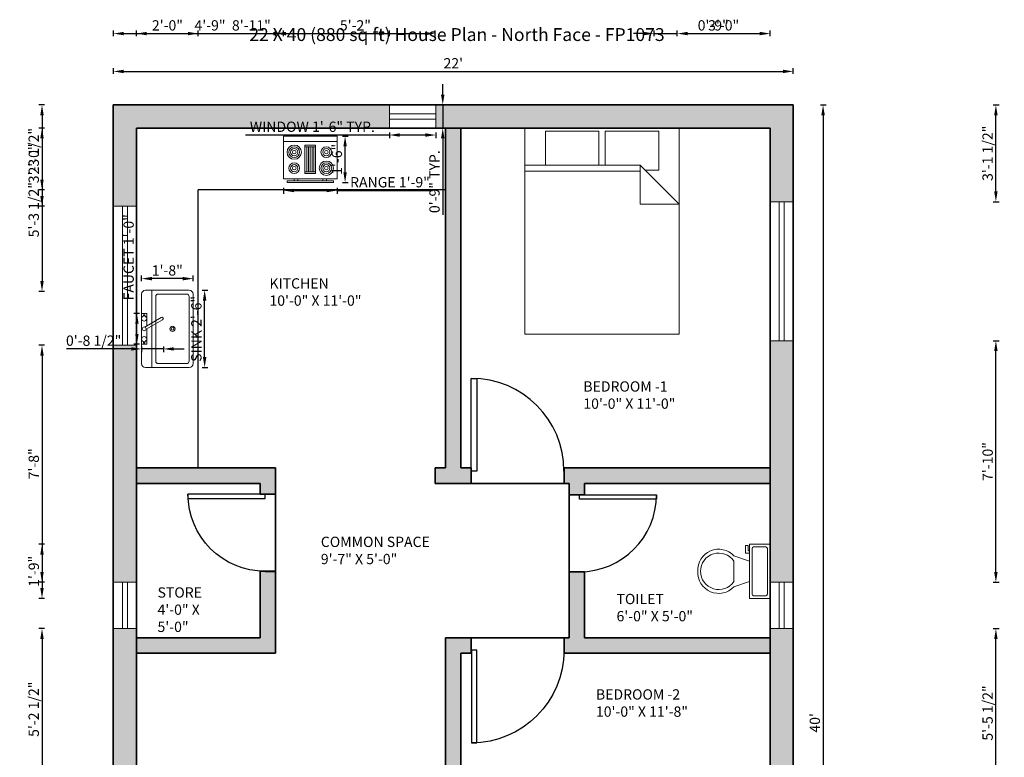
# Model space of a CAD drawing. Units: inches. Extents: x -34 to 348, y -513 to 46.
# Tile 2 of 2: x -34 to 348, y -240 to 46. Entities that reach past the tile are written whole.
import ezdxf

# ---------------------------------------------------------------- set-up
doc = ezdxf.new("R2010")
doc.units = ezdxf.units.IN
for name, color, linetype, lineweight in [('A-ANNO-DIMS', 2, 'Continuous', 18), ('A-ANNO-TEXT', 7, 'Continuous', 18), ('A-AREA-IDEN', 7, 'Continuous', 18), ('A-DOOR', 4, 'Continuous', 25), ('A-EQPM', 9, 'Continuous', 18), ('A-FLOR-CASE', 7, 'Continuous', 25), ('A-FLOR-FIXT', 8, 'Continuous', 18), ('A-FURN', 8, 'Continuous', 18), ('A-GLAZ', 6, 'Continuous', 18), ('A-WALL', 7, 'Continuous', 35), ('A-WALL-PATT', 251, 'Continuous', 13)]:
    doc.layers.add(name, color=color, linetype=linetype, lineweight=lineweight)
doc.styles.get("Standard").update_dxf_attribs({"font": 'arial.ttf'})
doc.dimstyles.new('ISO-25', dxfattribs={"dimtxt": 4, "dimasz": 4, "dimexe": 1.25, "dimexo": 0.625, "dimtad": 1, "dimlunit": 3, "dimtxsty": 'Standard', "dimcen": 2.5, "dimadec": 0, "dimazin": 0, "dimtfac": 1, "dimtmove": 0, "dimatfit": 3, "dimfxl": 1, "dimfxlon": 1, "dimarcsym": 0})

# ---------------------------------------------------------------- blocks, each defined once
blk = doc.blocks.new('*U2')
for p, q in [((9.5, -6), (9.5, -2)), ((-10, -8.5), (-8, -8.5)), ((-10, -9.5), (-10, -8.5)), ((-7, -9.5), (-10, -9.5)), ((-8, -8.5), (-8, -8)), ((-7, -8), (-7, -9.5)), ((-4, -8), (-6, -14)), ((4, -8), (6, -14)), ((4, -14), (-4, -14))]:
    blk.add_line(p, q)
blk.add_lwpolyline([(10.5, -8), (10.5, 0), (-10.5, 0), (-10.5, -8)], close=True)
for points in [[(-9.5, -2), (-9.5, -6)], [(8.5, -1), (-8.5, -1)], [(-8.5, -7), (8.5, -7)]]:
    blk.add_lwpolyline(points)
for centre, radius, start, end in [((-8.625, -1.875), 0.8839, 81.8699, 188.1301), ((8.625, -1.875), 0.8839, 351.8699, 98.1301), ((-8.625, -6.125), 0.8839, 171.869898, 278.1301), ((8.625, -6.125), 0.8839, 261.8699, 8.1301), ((-0.4772, -19.9188), 8.0953, 133.01722, 273.38), ((0.0374, -19.8731), 7.127, 124.50543, 269.7), ((-0.0373, -19.8731), 7.127, 270.3, 55.4946), ((0.4773, -19.9188), 8.0953, 266.62, 46.9828)]:
    blk.add_arc(centre, radius, start, end)
blk = doc.blocks.new('*U4')
for p, q in [((0, 0), (0, -100)), ((750, 0), (750, -100))]:
    blk.add_line(p, q)
blk.add_lwpolyline([(0, 0), (0, 750), (43.75, 750), (43.75, 0)], close=True)
blk.add_arc((0, 0), 750, 0, 90)
blk = doc.blocks.new('Sink-single - 30 in top')
blk.add_line((-15, -3.999996), (15, -3.999996))
for points in [[(-13.5, 0), (13.5, 0)], [(-15, -18.499996), (-15, -1.5)], [(15, -1.5), (15, -18.499996)], [(-13.5, -17.499996), (-13.5, -6.499996)], [(-12.5, -5.499996), (12.5, -5.499996)], [(13.5, -6.499996), (13.5, -17.499996)], [(12.5, -18.499996), (-12.5, -18.499996)], [(13.5, -19.999996), (-13.5, -19.999996)]]:
    blk.add_lwpolyline(points)
for radius in [1, 0.5]:
    blk.add_circle((0, -11.999996), radius)
for centre, radius, start, end in [((-13.5, -1.5), 1.5, 90, 180), ((13.5, -1.5), 1.5, 0, 90), ((-12.5, -6.499996), 1, 90, 180), ((12.5, -6.499996), 1, 0, 90), ((-13.5, -18.499996), 1.5, 180, 270), ((-12.5, -17.499996), 1, 180, 270), ((12.5, -17.499996), 1, 270, 0), ((13.5, -18.499996), 1.5, 270, 0)]:
    blk.add_arc(centre, radius, start, end)
blk = doc.blocks.new('Faucet - kit sink top')
for p, q in [((-5.5, -0.75), (-5.5, -1.25)), ((-4.94278, -0.75), (-5.5, -0.75)), ((-5.5, -1.25), (-4.94278, -1.25)), ((-0.14775, -1.7441), (3.56698, -8.1782)), ((4.43301, -7.6782), (0.71828, -1.2441)), ((4.94278, -0.75), (5.5, -0.75)), ((5.5, -1.25), (4.94278, -1.25)), ((5.5, -0.75), (5.5, -1.25))]:
    blk.add_line(p, q)
blk.add_lwpolyline([(-0.00587, -2), (-6, -2), (-6, 0), (6, 0), (6, -2), (1.15195, -2)])
for centre, radius in [((-4, -1), 1), ((4, -1), 1), ((0, -1), 0.75)]:
    blk.add_circle(centre, radius)
blk.add_arc((4, -7.9282), 0.5, 210, 30)
blk = doc.blocks.new('Range-Oven - 30 in top')
for p, q in [((0, -3), (30, -3)), ((12, -6), (18, -6)), ((13, -20), (13, -6)), ((14, -6), (14, -20)), ((15, -20), (15, -6)), ((16, -6), (16, -20)), ((17, -20), (17, -6)), ((18, -20), (12, -20)), ((6, -24), (6, -25)), ((8, -25), (8, -24)), ((22, -25), (22, -24)), ((24, -24), (24, -25))]:
    blk.add_line(p, q)
for points in [[(0, -24), (0, 0), (30, 0), (30, -24)], [(12, -21), (12, -5), (18, -5), (18, -21)], [(2, -26), (2, -25), (28, -25), (28, -26)]]:
    blk.add_lwpolyline(points, close=True)
for centre, radius in [((6, -9), 4), ((6, -9), 3), ((6, -9), 2), ((6, -9), 1), ((24, -9), 3), ((24, -9), 2), ((24, -9), 1), ((6, -18), 3), ((6, -18), 2), ((24, -18), 4), ((24, -18), 3), ((24, -18), 2), ((6, -18), 1), ((24, -18), 1)]:
    blk.add_circle(centre, radius)
blk = doc.blocks.new('Bed - Queen')
for p, q in [((0, -80.00003), (0, 0)), ((0, 0), (59.99999, 0)), ((59.99999, 0), (59.99999, -80.00003)), ((7.99999, -1.2), (28.79998, -1.2)), ((7.99999, -14.4), (7.99999, -1.2)), ((28.79998, -1.2), (28.79998, -14.4)), ((31.19999, -1.2), (51.99999, -1.2)), ((31.19999, -14.4), (31.19999, -1.2)), ((51.99999, -1.2), (51.99999, -16.4)), ((0, -14.4), (44.8, -14.4)), ((59.99999, -29.6), (44.8, -14.4)), ((44.8, -14.4), (44.8, -29.6)), ((44.8, -16.8), (0, -16.8)), ((51.99999, -16.4), (46.79936, -16.4)), ((44.8, -29.6), (59.99999, -29.6)), ((59.99999, -80.00003), (0, -80.00003))]:
    blk.add_line(p, q)
blk = doc.blocks.new('*D12')
at = {"layer": 'A-ANNO-DIMS', "color": 0, "lineweight": -2, "transparency": 16777216}
for p, q in [((2.13, 25.41), (2.13, 27.66)), ((266.13, 25.41), (266.13, 27.66)), ((6.13, 26.41), (262.13, 26.41))]:
    blk.add_line(p, q, dxfattribs=at)
at = {"layer": 'A-ANNO-DIMS', "color": 0, "transparency": 16777216}
for points in [[(6.13, 27.07), (6.13, 25.74), (2.13, 26.41)], [(262.13, 27.07), (262.13, 25.74), (266.13, 26.41)]]:
    blk.add_solid(points, dxfattribs=at)
at = {"layer": 'Defpoints', "color": 0, "transparency": 16777216}
for p in [(266.13, 26.41), (2.13, 13.4), (266.13, 13.4)]:
    blk.add_point(p, dxfattribs=at)
at = {"layer": 'A-ANNO-DIMS', "color": 0, "transparency": 16777216, "insert": (134.13, 29.04), "char_height": 4, "attachment_point": 5}
blk.add_mtext("22'", dxfattribs=at)
blk = doc.blocks.new('*D13')
at = {"layer": 'A-ANNO-DIMS', "color": 0, "lineweight": -2, "transparency": 16777216}
for p, q in [((276.72, 13.4), (278.97, 13.4)), ((277.72, 9.4), (277.72, -462.6)), ((276.72, -466.6), (278.97, -466.6))]:
    blk.add_line(p, q, dxfattribs=at)
at = {"layer": 'A-ANNO-DIMS', "color": 0, "transparency": 16777216}
for points in [[(277.06, 9.4), (278.39, 9.4), (277.72, 13.4)], [(277.06, -462.6), (278.39, -462.6), (277.72, -466.6)]]:
    blk.add_solid(points, dxfattribs=at)
at = {"layer": 'Defpoints', "color": 0, "transparency": 16777216}
for p in [(266.13, 13.4), (266.13, -466.6), (277.72, -466.6)]:
    blk.add_point(p, dxfattribs=at)
at = {"layer": 'A-ANNO-DIMS', "color": 0, "transparency": 16777216, "insert": (275.05, -226.6), "char_height": 4, "attachment_point": 5, "rotation": 90}
blk.add_mtext("40'", dxfattribs=at)
blk = doc.blocks.new('WIN-54IN')
for p, q in [((3.5, 54), (3.5, 0)), ((5.5, 54), (5.5, 0))]:
    blk.add_line(p, q)
blk.add_lwpolyline([(0, 54), (9, 54), (9, 0), (0, 0)], close=True)
blk = doc.blocks.new('WIN-18IN')
for p, q in [((3.5, 18), (3.5, 0)), ((5.5, 18), (5.5, 0))]:
    blk.add_line(p, q)
blk.add_lwpolyline([(0, 18), (9, 18), (9, 0), (0, 0)], close=True)
blk = doc.blocks.new('*D18')
at = {"layer": 'A-ANNO-DIMS', "color": 0, "lineweight": -2, "transparency": 16777216}
for p, q in [((109.34, 1.7), (53.47, 1.7)), ((109.34, 2.7), (109.34, 0.45)), ((123.34, 1.7), (113.34, 1.7)), ((127.34, 2.7), (127.34, 0.45))]:
    blk.add_line(p, q, dxfattribs=at)
at = {"layer": 'A-ANNO-DIMS', "color": 0, "transparency": 16777216}
for points in [[(113.34, 2.37), (113.34, 1.04), (109.34, 1.7)], [(123.34, 2.37), (123.34, 1.04), (127.34, 1.7)]]:
    blk.add_solid(points, dxfattribs=at)
at = {"layer": 'Defpoints', "color": 0, "transparency": 16777216}
for p in [(109.34, 4.4), (127.34, 4.4), (109.34, 1.7)]:
    blk.add_point(p, dxfattribs=at)
at = {"layer": 'A-ANNO-DIMS', "color": 0, "transparency": 16777216, "insert": (79.41, 4.4), "char_height": 4, "attachment_point": 5}
blk.add_mtext('WINDOW 1\'-6" TYP.', dxfattribs=at)
blk = doc.blocks.new('*D19')
at = {"layer": 'A-ANNO-DIMS', "color": 0, "lineweight": -2, "transparency": 16777216}
for p, q in [((130.04, 17.4), (130.04, 21.4)), ((129.04, 13.4), (131.29, 13.4)), ((130.04, 13.4), (130.04, 4.4)), ((129.04, 4.4), (131.29, 4.4)), ((130.04, 0.4), (130.04, -29.23))]:
    blk.add_line(p, q, dxfattribs=at)
at = {"layer": 'A-ANNO-DIMS', "color": 0, "transparency": 16777216}
for points in [[(129.37, 17.4), (130.71, 17.4), (130.04, 13.4)], [(129.37, 0.4), (130.71, 0.4), (130.04, 4.4)]]:
    blk.add_solid(points, dxfattribs=at)
at = {"layer": 'Defpoints', "color": 0, "transparency": 16777216}
for p in [(127.34, 13.4), (127.34, 4.4), (130.04, 4.4)]:
    blk.add_point(p, dxfattribs=at)
at = {"layer": 'A-ANNO-DIMS', "color": 0, "transparency": 16777216, "insert": (127.37, -16.41), "char_height": 4, "attachment_point": 5, "rotation": 90}
blk.add_mtext('0\'-9" TYP.', dxfattribs=at)
blk = doc.blocks.new('*D22')
at = {"layer": 'A-ANNO-DIMS', "color": 0, "lineweight": -2, "transparency": 16777216}
for p, q in [((36.58, -58.57), (38.83, -58.57)), ((37.58, -84.57), (37.58, -62.57)), ((36.58, -88.57), (38.83, -88.57))]:
    blk.add_line(p, q, dxfattribs=at)
at = {"layer": 'A-ANNO-DIMS', "color": 0, "transparency": 16777216}
for points in [[(36.92, -62.57), (38.25, -62.57), (37.58, -58.57)], [(36.92, -84.57), (38.25, -84.57), (37.58, -88.57)]]:
    blk.add_solid(points, dxfattribs=at)
at = {"layer": 'Defpoints', "color": 0, "transparency": 16777216}
for p in [(33.08, -58.57), (37.58, -58.57), (33.08, -88.57)]:
    blk.add_point(p, dxfattribs=at)
at = {"layer": 'A-ANNO-DIMS', "color": 0, "transparency": 16777216, "insert": (34.89, -73.57), "char_height": 4, "attachment_point": 5, "rotation": 90}
blk.add_mtext('SINK 2\'-6"', dxfattribs=at)
blk = doc.blocks.new('*D23')
at = {"layer": 'A-ANNO-DIMS', "color": 0, "lineweight": -2, "transparency": 16777216}
for p, q in [((13.08, -55.07), (13.08, -52.82)), ((33.08, -55.07), (33.08, -52.82)), ((29.08, -54.07), (17.08, -54.07))]:
    blk.add_line(p, q, dxfattribs=at)
at = {"layer": 'A-ANNO-DIMS', "color": 0, "transparency": 16777216}
for points in [[(17.08, -53.41), (17.08, -54.74), (13.08, -54.07)], [(29.08, -53.41), (29.08, -54.74), (33.08, -54.07)]]:
    blk.add_solid(points, dxfattribs=at)
at = {"layer": 'Defpoints', "color": 0, "transparency": 16777216}
for p in [(13.08, -54.07), (13.08, -58.57), (33.08, -58.57)]:
    blk.add_point(p, dxfattribs=at)
at = {"layer": 'A-ANNO-DIMS', "color": 0, "transparency": 16777216, "insert": (23.08, -51.41), "char_height": 4, "attachment_point": 5}
blk.add_mtext('1\'-8"', dxfattribs=at)
blk = doc.blocks.new('*D24')
at = {"layer": 'A-ANNO-DIMS', "color": 0, "lineweight": -2, "transparency": 16777216}
for p, q in [((11.28, -67.57), (11.28, -28.01)), ((12.28, -67.57), (10.03, -67.57)), ((11.28, -75.57), (11.28, -71.57)), ((12.28, -79.57), (10.03, -79.57))]:
    blk.add_line(p, q, dxfattribs=at)
at = {"layer": 'A-ANNO-DIMS', "color": 0, "transparency": 16777216}
for points in [[(10.62, -71.57), (11.95, -71.57), (11.28, -67.57)], [(10.62, -75.57), (11.95, -75.57), (11.28, -79.57)]]:
    blk.add_solid(points, dxfattribs=at)
at = {"layer": 'Defpoints', "color": 0, "transparency": 16777216}
for p in [(11.28, -67.57), (13.08, -67.57), (13.08, -79.57)]:
    blk.add_point(p, dxfattribs=at)
at = {"layer": 'A-ANNO-DIMS', "color": 0, "transparency": 16777216, "insert": (8.59, -45.79), "char_height": 4, "attachment_point": 5, "rotation": 90}
blk.add_mtext('FAUCET 1\'-0"', dxfattribs=at)
blk = doc.blocks.new('*D25')
at = {"layer": 'A-ANNO-DIMS', "color": 0, "lineweight": -2, "transparency": 16777216}
for p, q in [((9.08, -81.37), (-16.12, -81.37)), ((13.08, -80.37), (13.08, -82.62)), ((21.58, -81.37), (13.08, -81.37)), ((21.58, -80.37), (21.58, -82.62)), ((25.58, -81.37), (29.58, -81.37))]:
    blk.add_line(p, q, dxfattribs=at)
at = {"layer": 'A-ANNO-DIMS', "color": 0, "transparency": 16777216}
for points in [[(9.08, -80.71), (9.08, -82.04), (13.08, -81.37)], [(25.58, -80.71), (25.58, -82.04), (21.58, -81.37)]]:
    blk.add_solid(points, dxfattribs=at)
at = {"layer": 'Defpoints', "color": 0, "transparency": 16777216}
for p in [(13.08, -79.57), (21.58, -79.57), (13.08, -81.37)]:
    blk.add_point(p, dxfattribs=at)
at = {"layer": 'A-ANNO-DIMS', "color": 0, "transparency": 16777216, "insert": (-5.52, -78.68), "char_height": 4, "attachment_point": 5}
blk.add_mtext('0\'-8 1/2"', dxfattribs=at)
blk = doc.blocks.new('*D26')
at = {"layer": 'A-ANNO-DIMS', "color": 0, "lineweight": -2, "transparency": 16777216}
for p, q in [((68.22, -18.84), (68.22, -21.09)), ((89, -18.84), (89, -21.09)), ((72.22, -19.84), (85, -19.84)), ((89, -19.84), (126.1, -19.84))]:
    blk.add_line(p, q, dxfattribs=at)
at = {"layer": 'A-ANNO-DIMS', "color": 0, "transparency": 16777216}
for points in [[(72.22, -19.18), (72.22, -20.51), (68.22, -19.84)], [(85, -19.18), (85, -20.51), (89, -19.84)]]:
    blk.add_solid(points, dxfattribs=at)
at = {"layer": 'Defpoints', "color": 0, "transparency": 16777216}
for p in [(68.22, -16.73), (89, -16.73), (89, -19.84)]:
    blk.add_point(p, dxfattribs=at)
at = {"layer": 'A-ANNO-DIMS', "color": 0, "transparency": 16777216, "insert": (109.55, -17.15), "char_height": 4, "attachment_point": 5}
blk.add_mtext('RANGE 1\'-9"', dxfattribs=at)
blk = doc.blocks.new('*D27')
at = {"layer": 'A-ANNO-DIMS', "color": 0, "lineweight": -2, "transparency": 16777216}
for p, q in [((91.12, 1.29), (93.37, 1.29)), ((92.12, -12.73), (92.12, -2.71)), ((91.12, -16.73), (93.37, -16.73))]:
    blk.add_line(p, q, dxfattribs=at)
at = {"layer": 'A-ANNO-DIMS', "color": 0, "transparency": 16777216}
for points in [[(91.45, -2.71), (92.78, -2.71), (92.12, 1.29)], [(91.45, -12.73), (92.78, -12.73), (92.12, -16.73)]]:
    blk.add_solid(points, dxfattribs=at)
at = {"layer": 'Defpoints', "color": 0, "transparency": 16777216}
for p in [(89, 1.29), (92.12, 1.29), (89, -16.73)]:
    blk.add_point(p, dxfattribs=at)
at = {"layer": 'A-ANNO-DIMS', "color": 0, "transparency": 16777216, "insert": (89.45, -7.72), "char_height": 4, "attachment_point": 5, "rotation": 90}
blk.add_mtext('1\'-6"', dxfattribs=at)
blk = doc.blocks.new('*D33')
at = {"layer": 'A-ANNO-DIMS', "color": 0, "lineweight": -2, "transparency": 16777216}
for p, q in [((31.1, -510.8), (31.1, -513.05)), ((35.1, -511.8), (57.12, -511.8)), ((61.12, -510.8), (61.12, -513.05))]:
    blk.add_line(p, q, dxfattribs=at)
at = {"layer": 'A-ANNO-DIMS', "color": 0, "transparency": 16777216}
for points in [[(35.1, -511.13), (35.1, -512.47), (31.1, -511.8)], [(57.12, -511.13), (57.12, -512.47), (61.12, -511.8)]]:
    blk.add_solid(points, dxfattribs=at)
at = {"layer": 'Defpoints', "color": 0, "transparency": 16777216}
for p in [(31.1, -137.74), (61.12, -137.74), (61.12, -511.8)]:
    blk.add_point(p, dxfattribs=at)
at = {"layer": 'A-ANNO-DIMS', "color": 0, "transparency": 16777216, "insert": (46.11, -509.13), "char_height": 4, "attachment_point": 5}
blk.add_mtext('2\'-6"', dxfattribs=at)
blk = doc.blocks.new('*D34')
at = {"layer": 'A-ANNO-DIMS', "color": 0, "lineweight": -2, "transparency": 16777216}
for p, q in [((11.13, 40.1), (11.13, 42.35)), ((35.13, 40.1), (35.13, 42.35)), ((15.13, 41.1), (31.13, 41.1))]:
    blk.add_line(p, q, dxfattribs=at)
at = {"layer": 'A-ANNO-DIMS', "color": 0, "transparency": 16777216}
for points in [[(15.13, 41.77), (15.13, 40.44), (11.13, 41.1)], [(31.13, 41.77), (31.13, 40.44), (35.13, 41.1)]]:
    blk.add_solid(points, dxfattribs=at)
at = {"layer": 'Defpoints', "color": 0, "transparency": 16777216}
for p in [(35.13, 41.1), (11.13, -127.6), (35.13, -127.6)]:
    blk.add_point(p, dxfattribs=at)
at = {"layer": 'A-ANNO-DIMS', "color": 0, "transparency": 16777216, "insert": (23.13, 43.77), "char_height": 4, "attachment_point": 5}
blk.add_mtext('2\'-0"', dxfattribs=at)
blk = doc.blocks.new('*D35')
at = {"layer": 'A-ANNO-DIMS', "color": 0, "lineweight": -2, "transparency": 16777216}
for p, q in [((-24.57, 4.4), (-26.82, 4.4)), ((-25.57, 0.4), (-25.57, -15.6)), ((-24.57, -19.6), (-26.82, -19.6))]:
    blk.add_line(p, q, dxfattribs=at)
at = {"layer": 'A-ANNO-DIMS', "color": 0, "transparency": 16777216}
for points in [[(-26.24, 0.4), (-24.91, 0.4), (-25.57, 4.4)], [(-26.24, -15.6), (-24.91, -15.6), (-25.57, -19.6)]]:
    blk.add_solid(points, dxfattribs=at)
at = {"layer": 'Defpoints', "color": 0, "transparency": 16777216}
for p in [(131.13, 4.4), (-25.57, -19.6), (131.13, -19.6)]:
    blk.add_point(p, dxfattribs=at)
at = {"layer": 'A-ANNO-DIMS', "color": 0, "transparency": 16777216, "insert": (-28.24, -7.6), "char_height": 4, "attachment_point": 5, "rotation": 90}
blk.add_mtext('2\'-0"', dxfattribs=at)
blk = doc.blocks.new('*D36')
at = {"layer": 'A-ANNO-DIMS', "color": 0, "lineweight": -2, "transparency": 16777216}
for p, q in [((11.13, 40.1), (11.13, 42.35)), ((68.22, 40.1), (68.22, 42.35)), ((15.13, 41.1), (64.22, 41.1))]:
    blk.add_line(p, q, dxfattribs=at)
at = {"layer": 'A-ANNO-DIMS', "color": 0, "transparency": 16777216}
for points in [[(15.13, 41.77), (15.13, 40.44), (11.13, 41.1)], [(64.22, 41.77), (64.22, 40.44), (68.22, 41.1)]]:
    blk.add_solid(points, dxfattribs=at)
at = {"layer": 'Defpoints', "color": 0, "transparency": 16777216}
for p in [(68.22, 41.1), (11.13, 4.4), (68.22, 1.29)]:
    blk.add_point(p, dxfattribs=at)
at = {"layer": 'A-ANNO-DIMS', "color": 0, "transparency": 16777216, "insert": (39.67, 43.77), "char_height": 4, "attachment_point": 5}
blk.add_mtext('4\'-9"', dxfattribs=at)
blk = doc.blocks.new('*D37')
at = {"layer": 'A-ANNO-DIMS', "color": 0, "lineweight": -2, "transparency": 16777216}
for p, q in [((-24.57, 4.4), (-26.82, 4.4)), ((-25.57, 0.4), (-25.57, -55.01)), ((-24.57, -59.01), (-26.82, -59.01))]:
    blk.add_line(p, q, dxfattribs=at)
at = {"layer": 'A-ANNO-DIMS', "color": 0, "transparency": 16777216}
for points in [[(-26.24, 0.4), (-24.91, 0.4), (-25.57, 4.4)], [(-26.24, -55.01), (-24.91, -55.01), (-25.57, -59.01)]]:
    blk.add_solid(points, dxfattribs=at)
at = {"layer": 'Defpoints', "color": 0, "transparency": 16777216}
for p in [(11.13, 4.4), (-25.57, -59.01), (13.52, -59.01)]:
    blk.add_point(p, dxfattribs=at)
at = {"layer": 'A-ANNO-DIMS', "color": 0, "transparency": 16777216, "insert": (-28.27, -27.3), "char_height": 4, "attachment_point": 5, "rotation": 90}
blk.add_mtext('5\'-3 1/2"', dxfattribs=at)
blk = doc.blocks.new('*D38')
at = {"layer": 'A-ANNO-DIMS', "color": 0, "lineweight": -2, "transparency": 16777216}
for p, q in [((2.13, 40.1), (2.13, 42.35)), ((109.34, 40.1), (109.34, 42.35)), ((6.13, 41.1), (105.34, 41.1))]:
    blk.add_line(p, q, dxfattribs=at)
at = {"layer": 'A-ANNO-DIMS', "color": 0, "transparency": 16777216}
for points in [[(6.13, 41.77), (6.13, 40.44), (2.13, 41.1)], [(105.34, 41.77), (105.34, 40.44), (109.34, 41.1)]]:
    blk.add_solid(points, dxfattribs=at)
at = {"layer": 'Defpoints', "color": 0, "transparency": 16777216}
for p in [(109.34, 41.1), (2.13, 13.4), (109.34, 13.4)]:
    blk.add_point(p, dxfattribs=at)
at = {"layer": 'A-ANNO-DIMS', "color": 0, "transparency": 16777216, "insert": (55.73, 43.77), "char_height": 4, "attachment_point": 5}
blk.add_mtext('8\'-11"', dxfattribs=at)
blk = doc.blocks.new('*D39')
at = {"layer": 'A-ANNO-DIMS', "color": 0, "lineweight": -2, "transparency": 16777216}
for p, q in [((-24.57, 13.4), (-26.82, 13.4)), ((-25.57, 9.4), (-25.57, -21.97)), ((-24.57, -25.97), (-26.82, -25.97))]:
    blk.add_line(p, q, dxfattribs=at)
at = {"layer": 'A-ANNO-DIMS', "color": 0, "transparency": 16777216}
for points in [[(-26.24, 9.4), (-24.91, 9.4), (-25.57, 13.4)], [(-26.24, -21.97), (-24.91, -21.97), (-25.57, -25.97)]]:
    blk.add_solid(points, dxfattribs=at)
at = {"layer": 'Defpoints', "color": 0, "transparency": 16777216}
for p in [(2.13, 13.4), (-25.57, -25.97), (2.13, -25.97)]:
    blk.add_point(p, dxfattribs=at)
at = {"layer": 'A-ANNO-DIMS', "color": 0, "transparency": 16777216, "insert": (-28.27, -6.28), "char_height": 4, "attachment_point": 5, "rotation": 90}
blk.add_mtext('3\'-3 1/2"', dxfattribs=at)
blk = doc.blocks.new('*D40')
at = {"layer": 'A-ANNO-DIMS', "color": 0, "lineweight": -2, "transparency": 16777216}
for p, q in [((-24.57, -79.97), (-26.82, -79.97)), ((-25.57, -83.97), (-25.57, -168.01)), ((-24.57, -172.01), (-26.82, -172.01))]:
    blk.add_line(p, q, dxfattribs=at)
at = {"layer": 'A-ANNO-DIMS', "color": 0, "transparency": 16777216}
for points in [[(-26.24, -83.97), (-24.91, -83.97), (-25.57, -79.97)], [(-26.24, -168.01), (-24.91, -168.01), (-25.57, -172.01)]]:
    blk.add_solid(points, dxfattribs=at)
at = {"layer": 'Defpoints', "color": 0, "transparency": 16777216}
for p in [(2.13, -79.97), (-25.57, -172.01), (2.13, -172.01)]:
    blk.add_point(p, dxfattribs=at)
at = {"layer": 'A-ANNO-DIMS', "color": 0, "transparency": 16777216, "insert": (-28.24, -125.99), "char_height": 4, "attachment_point": 5, "rotation": 90}
blk.add_mtext('7\'-8"', dxfattribs=at)
blk = doc.blocks.new('*D41')
at = {"layer": 'A-ANNO-DIMS', "color": 0, "lineweight": -2, "transparency": 16777216}
for p, q in [((-24.57, -190.01), (-26.82, -190.01)), ((-25.57, -194.01), (-25.57, -248.61)), ((-24.57, -252.61), (-26.82, -252.61))]:
    blk.add_line(p, q, dxfattribs=at)
at = {"layer": 'A-ANNO-DIMS', "color": 0, "transparency": 16777216}
for points in [[(-26.24, -194.01), (-24.91, -194.01), (-25.57, -190.01)], [(-26.24, -248.61), (-24.91, -248.61), (-25.57, -252.61)]]:
    blk.add_solid(points, dxfattribs=at)
at = {"layer": 'Defpoints', "color": 0, "transparency": 16777216}
for p in [(2.13, -190.01), (-25.57, -252.61), (2.13, -252.61)]:
    blk.add_point(p, dxfattribs=at)
at = {"layer": 'A-ANNO-DIMS', "color": 0, "transparency": 16777216, "insert": (-28.27, -221.31), "char_height": 4, "attachment_point": 5, "rotation": 90}
blk.add_mtext('5\'-2 1/2"', dxfattribs=at)
blk = doc.blocks.new('*D43')
at = {"layer": 'A-ANNO-DIMS', "color": 0, "lineweight": -2, "transparency": 16777216}
for p, q in [((343.83, 13.4), (346.08, 13.4)), ((344.83, -20.18), (344.83, 9.4)), ((343.83, -24.18), (346.08, -24.18))]:
    blk.add_line(p, q, dxfattribs=at)
at = {"layer": 'A-ANNO-DIMS', "color": 0, "transparency": 16777216}
for points in [[(344.16, 9.4), (345.49, 9.4), (344.83, 13.4)], [(344.16, -20.18), (345.49, -20.18), (344.83, -24.18)]]:
    blk.add_solid(points, dxfattribs=at)
at = {"layer": 'Defpoints', "color": 0, "transparency": 16777216}
for p in [(266.13, 13.4), (344.83, 13.4), (266.13, -24.18)]:
    blk.add_point(p, dxfattribs=at)
at = {"layer": 'A-ANNO-DIMS', "color": 0, "transparency": 16777216, "insert": (342.13, -5.39), "char_height": 4, "attachment_point": 5, "rotation": 90}
blk.add_mtext('3\'-1 1/2"', dxfattribs=at)
blk = doc.blocks.new('*D44')
at = {"layer": 'A-ANNO-DIMS', "color": 0, "lineweight": -2, "transparency": 16777216}
for p, q in [((343.83, -78.18), (346.08, -78.18)), ((344.83, -168.01), (344.83, -82.18)), ((343.83, -172.01), (346.08, -172.01))]:
    blk.add_line(p, q, dxfattribs=at)
at = {"layer": 'A-ANNO-DIMS', "color": 0, "transparency": 16777216}
for points in [[(344.16, -82.18), (345.49, -82.18), (344.83, -78.18)], [(344.16, -168.01), (345.49, -168.01), (344.83, -172.01)]]:
    blk.add_solid(points, dxfattribs=at)
at = {"layer": 'Defpoints', "color": 0, "transparency": 16777216}
for p in [(266.13, -78.18), (344.83, -78.18), (266.13, -172.01)]:
    blk.add_point(p, dxfattribs=at)
at = {"layer": 'A-ANNO-DIMS', "color": 0, "transparency": 16777216, "insert": (342.16, -125.1), "char_height": 4, "attachment_point": 5, "rotation": 90}
blk.add_mtext('7\'-10"', dxfattribs=at)
blk = doc.blocks.new('*D45')
at = {"layer": 'A-ANNO-DIMS', "color": 0, "lineweight": -2, "transparency": 16777216}
for p, q in [((343.83, -190.01), (346.08, -190.01)), ((344.83, -251.53), (344.83, -194.01)), ((343.83, -255.53), (346.08, -255.53))]:
    blk.add_line(p, q, dxfattribs=at)
at = {"layer": 'A-ANNO-DIMS', "color": 0, "transparency": 16777216}
for points in [[(344.16, -194.01), (345.49, -194.01), (344.83, -190.01)], [(344.16, -251.53), (345.49, -251.53), (344.83, -255.53)]]:
    blk.add_solid(points, dxfattribs=at)
at = {"layer": 'Defpoints', "color": 0, "transparency": 16777216}
for p in [(266.13, -190.01), (344.83, -190.01), (266.13, -255.53)]:
    blk.add_point(p, dxfattribs=at)
at = {"layer": 'A-ANNO-DIMS', "color": 0, "transparency": 16777216, "insert": (342.13, -222.77), "char_height": 4, "attachment_point": 5, "rotation": 90}
blk.add_mtext('5\'-5 1/2"', dxfattribs=at)
blk = doc.blocks.new('*D48')
at = {"layer": 'A-ANNO-DIMS', "color": 0, "lineweight": -2, "transparency": 16777216}
for p, q in [((-24.57, -157.24), (-26.82, -157.24)), ((-25.57, -161.24), (-25.57, -174.24)), ((-24.57, -178.24), (-26.82, -178.24))]:
    blk.add_line(p, q, dxfattribs=at)
at = {"layer": 'A-ANNO-DIMS', "color": 0, "transparency": 16777216}
for points in [[(-26.24, -161.24), (-24.91, -161.24), (-25.57, -157.24)], [(-26.24, -174.24), (-24.91, -174.24), (-25.57, -178.24)]]:
    blk.add_solid(points, dxfattribs=at)
at = {"layer": 'Defpoints', "color": 0, "transparency": 16777216}
for p in [(249.13, -157.24), (-25.57, -178.24), (249.13, -178.24)]:
    blk.add_point(p, dxfattribs=at)
at = {"layer": 'A-ANNO-DIMS', "color": 0, "transparency": 16777216, "insert": (-28.24, -167.74), "char_height": 4, "attachment_point": 5, "rotation": 90}
blk.add_mtext('1\'-9"', dxfattribs=at)
blk = doc.blocks.new('*D49')
at = {"layer": 'A-ANNO-DIMS', "color": 0, "lineweight": -2, "transparency": 16777216}
for p, q in [((229.13, -510.8), (229.13, -513.05)), ((233.13, -511.8), (253.13, -511.8)), ((257.13, -510.8), (257.13, -513.05))]:
    blk.add_line(p, q, dxfattribs=at)
at = {"layer": 'A-ANNO-DIMS', "color": 0, "transparency": 16777216}
for points in [[(233.13, -511.13), (233.13, -512.47), (229.13, -511.8)], [(253.13, -511.13), (253.13, -512.47), (257.13, -511.8)]]:
    blk.add_solid(points, dxfattribs=at)
at = {"layer": 'Defpoints', "color": 0, "transparency": 16777216}
for p in [(229.13, -167.74), (257.13, -178.24), (257.13, -511.8)]:
    blk.add_point(p, dxfattribs=at)
at = {"layer": 'A-ANNO-DIMS', "color": 0, "transparency": 16777216, "insert": (243.13, -509.17), "char_height": 4, "attachment_point": 5}
blk.add_mtext('2\'-4"', dxfattribs=at)
blk = doc.blocks.new('*D50')
at = {"layer": 'A-ANNO-DIMS', "color": 0, "lineweight": -2, "transparency": 16777216}
for p, q in [((221.89, -510.8), (221.89, -513.05)), ((225.89, -511.8), (253.13, -511.8)), ((257.13, -510.8), (257.13, -513.05))]:
    blk.add_line(p, q, dxfattribs=at)
at = {"layer": 'A-ANNO-DIMS', "color": 0, "transparency": 16777216}
for points in [[(225.89, -511.13), (225.89, -512.47), (221.89, -511.8)], [(253.13, -511.13), (253.13, -512.47), (257.13, -511.8)]]:
    blk.add_solid(points, dxfattribs=at)
at = {"layer": 'Defpoints', "color": 0, "transparency": 16777216}
for p in [(221.89, 4.4), (257.13, 4.4), (257.13, -511.8)]:
    blk.add_point(p, dxfattribs=at)
at = {"layer": 'A-ANNO-DIMS', "color": 0, "transparency": 16777216, "insert": (239.51, -509.17), "char_height": 4, "attachment_point": 5}
blk.add_mtext('2\'-11"', dxfattribs=at)
blk = doc.blocks.new('*D51')
at = {"layer": 'A-ANNO-DIMS', "color": 0, "lineweight": -2, "transparency": 16777216}
for p, q in [((221.13, 40.1), (221.13, 42.35)), ((257.13, 40.1), (257.13, 42.35)), ((225.13, 41.1), (253.13, 41.1))]:
    blk.add_line(p, q, dxfattribs=at)
at = {"layer": 'A-ANNO-DIMS', "color": 0, "transparency": 16777216}
for points in [[(225.13, 41.77), (225.13, 40.44), (221.13, 41.1)], [(253.13, 41.77), (253.13, 40.44), (257.13, 41.1)]]:
    blk.add_solid(points, dxfattribs=at)
at = {"layer": 'Defpoints', "color": 0, "transparency": 16777216}
for p in [(257.13, 41.1), (221.13, -343.93), (257.13, -343.93)]:
    blk.add_point(p, dxfattribs=at)
at = {"layer": 'A-ANNO-DIMS', "color": 0, "transparency": 16777216, "insert": (239.13, 43.77), "char_height": 4, "attachment_point": 5}
blk.add_mtext('3\'-0"', dxfattribs=at)
blk = doc.blocks.new('*D52')
at = {"layer": 'A-ANNO-DIMS', "color": 0, "lineweight": -2, "transparency": 16777216}
for p, q in [((65.13, 40.1), (65.13, 42.35)), ((127.13, 40.1), (127.13, 42.35)), ((69.13, 41.1), (123.13, 41.1))]:
    blk.add_line(p, q, dxfattribs=at)
at = {"layer": 'A-ANNO-DIMS', "color": 0, "transparency": 16777216}
for points in [[(69.13, 41.77), (69.13, 40.44), (65.13, 41.1)], [(123.13, 41.77), (123.13, 40.44), (127.13, 41.1)]]:
    blk.add_solid(points, dxfattribs=at)
at = {"layer": 'Defpoints', "color": 0, "transparency": 16777216}
for p in [(127.13, 41.1), (65.13, -127.6), (127.13, -127.6)]:
    blk.add_point(p, dxfattribs=at)
at = {"layer": 'A-ANNO-DIMS', "color": 0, "transparency": 16777216, "insert": (96.13, 43.77), "char_height": 4, "attachment_point": 5}
blk.add_mtext('5\'-2"', dxfattribs=at)
blk = doc.blocks.new('*D53')
at = {"layer": 'A-ANNO-DIMS', "color": 0, "lineweight": -2, "transparency": 16777216}
for p, q in [((212.09, 40.1), (212.09, 42.35)), ((221.13, 40.1), (221.13, 42.35)), ((208.09, 41.1), (204.09, 41.1)), ((212.09, 41.1), (221.13, 41.1)), ((225.13, 41.1), (241.01, 41.1))]:
    blk.add_line(p, q, dxfattribs=at)
at = {"layer": 'A-ANNO-DIMS', "color": 0, "transparency": 16777216}
for points in [[(208.09, 41.77), (208.09, 40.44), (212.09, 41.1)], [(225.13, 41.77), (225.13, 40.44), (221.13, 41.1)]]:
    blk.add_solid(points, dxfattribs=at)
at = {"layer": 'Defpoints', "color": 0, "transparency": 16777216}
for p in [(221.13, 41.1), (212.09, -343.93), (221.13, -343.93)]:
    blk.add_point(p, dxfattribs=at)
at = {"layer": 'A-ANNO-DIMS', "color": 0, "transparency": 16777216, "insert": (235.07, 43.77), "char_height": 4, "attachment_point": 5}
blk.add_mtext('0\'-9"', dxfattribs=at)

msp = doc.modelspace()

# ---------------------------------------------------------------- hatches: boundary and pattern name
at = {"layer": 'A-WALL-PATT'}
h = msp.add_hatch(color=256, dxfattribs=at)
h.dxf.hatch_style = 1
h.paths.add_polyline_path([(109.341, 13.405), (2.127, 13.405), (2.127, -25.971), (11.127, -25.971), (11.127, 4.405), (109.341, 4.405)])
h.paths.add_polyline_path([(266.127, 13.405), (127.341, 13.405), (127.341, 4.405), (131.127, 4.405), (137.127, 4.405), (257.127, 4.405), (257.127, -24.182), (266.127, -24.182)])
h.paths.add_polyline_path([(11.127, -79.971), (2.127, -79.971), (2.127, -172.013), (11.127, -172.013)])
h.paths.add_polyline_path([(65.127, -127.595), (11.127, -127.595), (11.127, -133.595), (59.127, -133.595), (59.127, -137.743), (61.124, -137.743), (65.127, -137.743), (65.127, -133.595)])
h.paths.add_polyline_path([(65.127, -167.764), (61.124, -167.764, -0.0092932), (60.008, -167.743), (59.127, -167.743), (59.127, -193.595), (11.127, -193.595), (11.127, -199.595), (59.127, -199.595), (65.127, -199.595)])
h.paths.add_polyline_path([(11.127, -190.013), (2.127, -190.013), (2.127, -252.614), (11.127, -252.614)])
h.paths.add_polyline_path([(11.127, -306.614), (2.127, -306.614), (2.127, -388.939), (11.127, -388.939)])
h.paths.add_polyline_path([(85.316, -461.006), (85.316, -460.595), (11.127, -460.595), (11.127, -466.595), (85.316, -466.595)])
h.paths.add_polyline_path([(11.127, -442.939), (2.127, -442.939), (2.127, -466.595), (11.127, -466.595)])
h.paths.add_polyline_path([(137.127, -427.93), (257.127, -427.93), (257.127, -421.93), (131.127, -421.93), (125.127, -421.93), (125.127, -427.93), (131.127, -427.93), (131.127, -460.595), (127.316, -460.595), (127.316, -466.595), (132.166, -466.595), (137.127, -466.595)])
h.paths.add_polyline_path([(266.127, -394.659), (257.127, -394.659), (257.127, -421.93), (257.127, -427.93), (266.127, -427.93)])
h.paths.add_polyline_path([(266.127, -309.532), (257.127, -309.532), (257.127, -343.93), (257.127, -360.659), (266.127, -360.659)])
h.paths.add_polyline_path([(257.127, -338.93), (137.127, -338.93), (137.127, -199.595), (141.127, -199.595), (141.127, -193.595), (131.127, -193.595), (131.127, -338.93), (127.127, -338.93), (127.127, -339.114), (127.127, -343.93), (137.127, -343.93), (257.127, -343.93)])
h.paths.add_polyline_path([(91.006, -338.93), (11.127, -338.93), (11.127, -343.93), (91.006, -343.93)])
h.paths.add_polyline_path([(266.127, -190.013), (257.127, -190.013), (257.127, -255.532), (266.127, -255.532)])
h.paths.add_polyline_path([(257.127, -193.595), (185.127, -193.595), (185.127, -167.989), (179.127, -167.989), (179.127, -193.595), (177.136, -193.595), (177.136, -198.391, -0.0057168), (177.127, -199.214), (177.127, -199.595), (179.127, -199.595), (185.127, -199.595), (257.127, -199.595)])
h.paths.add_polyline_path([(266.127, -78.182), (257.127, -78.182), (257.127, -172.013), (266.127, -172.013)])
h.paths.add_polyline_path([(257.127, -127.595), (177.127, -127.595), (177.127, -133.595), (179.127, -133.595), (179.127, -137.989), (183.118, -137.989), (185.127, -137.989), (185.127, -133.595), (257.127, -133.595)])
h.paths.add_polyline_path([(137.127, 4.405), (131.127, 4.405), (131.127, -127.595), (127.127, -127.595), (127.127, -133.595), (131.127, -133.595), (137.127, -133.595), (141.127, -133.595), (141.127, -128.797), (141.127, -127.595), (137.127, -127.595)])

# ---------------------------------------------------------------- linework, layer by layer
at = {"layer": 'A-FLOR-CASE'}
for p in [(131.127, -19.595), (35.127, -127.595)]:
    msp.add_line(p, (35.127, -19.595), dxfattribs=at)
at = {"layer": 'A-WALL'}
for p, q in [((2.127, 13.405), (266.127, 13.405)), ((2.127, -466.595), (2.127, 13.405)), ((266.127, 13.405), (266.127, -427.93)), ((11.127, 4.405), (131.127, 4.405)), ((11.127, -466.595), (11.127, 4.405)), ((131.127, 4.405), (137.127, 4.405)), ((131.127, -127.595), (131.127, 4.405)), ((137.127, 4.405), (257.127, 4.405)), ((137.127, -127.595), (137.127, 4.405)), ((257.127, 4.405), (257.127, -343.93)), ((11.127, -127.595), (65.127, -127.595)), ((65.127, -133.595), (65.127, -127.595)), ((127.127, -127.595), (127.127, -133.595)), ((127.127, -127.595), (131.127, -127.595)), ((137.127, -127.595), (141.127, -127.595)), ((141.127, -127.595), (141.127, -133.595)), ((177.127, -127.595), (177.127, -133.595)), ((177.127, -127.595), (257.127, -127.595)), ((11.127, -133.595), (59.127, -133.595)), ((59.127, -133.595), (59.127, -137.743)), ((65.127, -133.595), (65.127, -199.595)), ((127.127, -133.595), (131.127, -133.595)), ((137.127, -133.595), (131.127, -133.595)), ((137.127, -133.595), (179.127, -133.595)), ((179.127, -133.595), (179.127, -193.595)), ((185.127, -133.595), (185.127, -137.989)), ((185.127, -133.595), (257.127, -133.595)), ((65.127, -137.743), (59.127, -137.743)), ((185.127, -137.989), (179.127, -137.989)), ((65.127, -167.743), (59.127, -167.743)), ((59.127, -167.743), (59.127, -193.595)), ((185.127, -167.989), (179.127, -167.989)), ((185.127, -167.989), (185.127, -193.595)), ((59.127, -193.595), (11.127, -193.595)), ((179.127, -193.595), (131.127, -193.595)), ((131.127, -338.93), (131.127, -193.595)), ((141.127, -199.595), (141.127, -193.595)), ((177.127, -199.595), (177.127, -193.595)), ((185.127, -193.595), (257.127, -193.595)), ((59.127, -199.595), (11.127, -199.595)), ((59.127, -199.595), (65.127, -199.595)), ((141.127, -199.595), (137.127, -199.595)), ((137.127, -338.93), (137.127, -199.595)), ((179.127, -199.595), (177.127, -199.595)), ((185.127, -199.595), (179.127, -199.595)), ((185.127, -199.595), (257.127, -199.595))]:
    msp.add_line(p, q, dxfattribs=at)

# ---------------------------------------------------------------- block references
at = {"layer": 'A-DOOR', "xscale": 0.0479834075053935, "yscale": 0.0479834075053935, "zscale": 0.0479834075053935}
msp.add_blockref('*U4', (141.127, -128.797), dxfattribs=at)
at = {"layer": 'A-DOOR'}
for p, xscale, yscale, zscale, rotation in [((61.124, -137.743), -0.040027650715538, 0.040027650715538, 0.040027650715538, 90), ((183.118, -137.989), 0.0399172122118605, 0.0399172122118605, 0.0399172122118605, 270), ((141.142, -198.391), -0.0479923476985897, 0.0479923476985897, 0.0479923476985897, 180)]:
    msp.add_blockref('*U4', p, dxfattribs=dict(at, xscale=xscale, yscale=yscale, zscale=zscale, rotation=rotation))
at = {"layer": 'A-EQPM', "xscale": 0.6928203345745566, "yscale": 0.6928203345745566, "zscale": 0.6928203345745566}
msp.add_blockref('Range-Oven - 30 in top', (68.215, 1.287), dxfattribs=at)
at = {"layer": 'A-FLOR-FIXT'}
for name, p, rotation in [('Sink-single - 30 in top', (13.082, -73.575), 90), ('Faucet - kit sink top', (13.082, -73.575), 90), ('*U2', (257.127, -167.738), 270)]:
    msp.add_blockref(name, p, dxfattribs=dict(at, rotation=rotation))
at = {"layer": 'A-FURN'}
msp.add_blockref('Bed - Queen', (161.891, 4.405), dxfattribs=at)
at = {"layer": 'A-GLAZ', "extrusion": (0, 0, -1), "zscale": -1, "rotation": 270.0000000000002}
msp.add_blockref('WIN-18IN', (-127.341, 13.405), dxfattribs=at)
at = {"layer": 'A-GLAZ'}
for name, p in [('WIN-54IN', (2.127, -79.971)), ('WIN-54IN', (257.127, -78.182)), ('WIN-18IN', (2.127, -190.013)), ('WIN-18IN', (257.127, -190.013))]:
    msp.add_blockref(name, p, dxfattribs=at)

# ---------------------------------------------------------------- texts
at = {"layer": 'A-ANNO-TEXT', "insert": (54.926, 43.219), "char_height": 5, "attachment_point": 1}
msp.add_mtext_dynamic_manual_height_columns('22 X 40 (880 sq ft) House Plan - North Face - FP1073', width=228.37722, gutter_width=12.5, heights=[0], dxfattribs=at)
at = {"layer": 'A-AREA-IDEN', "char_height": 4, "attachment_point": 1}
for s, width, insert in [('KITCHEN\\P10\'-0" X 11\'-0"', 64.44418, (62.748, -53.933)), ('BEDROOM -1\\P10\'-0" X 11\'-0"', 61.1625, (184.634, -93.956)), ('COMMON SPACE\\P9\'-7" X 5\'-0"', 82.73794, (82.701, -154.301)), ('STORE\\P4\'-0" X 5\'-0"', 29.61025, (19.288, -173.973)), ('TOILET\\P6\'-0" X 5\'-0"', 30.90505, (197.522, -176.499)), ('BEDROOM -2\\P10\'-0" X 11\'-8"', 51.47015, (189.53, -213.565))]:
    msp.add_mtext_dynamic_manual_height_columns(s, width=width, gutter_width=12.5, heights=[0], dxfattribs=dict(at, insert=insert))

# ---------------------------------------------------------------- dimensions: what is measured, and where the dimension line sits
at = {"layer": 'A-ANNO-DIMS'}
for base, p1, p2, override, picture, middle in [((109.341, 41.105), (2.127, 13.405), (109.341, 13.405), {"dimdec": 1, "dimlfac": 1, "dimrnd": 0, "dimzin": 1, "dimdsep": 46, "dimlunit": 4, "dimfrac": 2}, '*D38', (55.734, 43.772)), ((35.127, 41.105), (11.127, -127.595), (35.127, -127.595), {"dimdec": 1, "dimlfac": 1, "dimrnd": 0, "dimzin": 1, "dimdsep": 46, "dimlunit": 4, "dimfrac": 2}, '*D34', (23.127, 43.772)), ((68.215, 41.105), (11.127, 4.405), (68.215, 1.287), {"dimdec": 1, "dimlfac": 1, "dimrnd": 0, "dimzin": 1, "dimdsep": 46, "dimlunit": 4, "dimfrac": 2}, '*D36', (39.671, 43.772)), ((127.127, 41.105), (65.127, -127.595), (127.127, -127.595), {"dimdec": 1, "dimlfac": 1, "dimrnd": 0, "dimzin": 1, "dimdsep": 46, "dimlunit": 4, "dimfrac": 2}, '*D52', (96.127, 43.772)), ((221.127, 41.105), (212.094, -343.93), (221.127, -343.93), {"dimdec": 1, "dimlfac": 1, "dimrnd": 0, "dimzin": 1, "dimdsep": 46, "dimlunit": 4, "dimfrac": 2}, '*D53', (235.068, 43.772)), ((257.127, 41.105), (221.127, -343.93), (257.127, -343.93), {"dimdec": 1, "dimlfac": 1, "dimrnd": 0, "dimzin": 1, "dimdsep": 46, "dimlunit": 4, "dimfrac": 2}, '*D51', (239.127, 43.773)), ((266.127, 26.405), (2.127, 13.405), (266.127, 13.405), {"dimclrd": 0, "dimclre": 0, "dimclrt": 0}, '*D12', (134.127, 29.038)), ((257.127, -511.8), (221.891, 4.405), (257.127, 4.405), {"dimdec": 1, "dimlfac": 1, "dimrnd": 0, "dimzin": 1, "dimdsep": 46, "dimlunit": 4, "dimfrac": 2}, '*D50', (239.509, -509.166)), ((61.124, -511.8), (31.103, -137.743), (61.124, -137.743), {"dimdec": 1, "dimlfac": 1, "dimrnd": 0, "dimzin": 1, "dimdsep": 46, "dimlunit": 4, "dimfrac": 2}, '*D33', (46.114, -509.132)), ((257.127, -511.8), (229.127, -167.738), (257.127, -178.238), {"dimdec": 1, "dimlfac": 1, "dimrnd": 0, "dimzin": 1, "dimdsep": 46, "dimlunit": 4, "dimfrac": 2}, '*D49', (243.127, -509.166))]:
    dim = msp.add_linear_dim(base=base, p1=p1, p2=p2, dimstyle='ISO-25', override=override, dxfattribs=at)
    dim.commit()
    dim.dimension.update_dxf_attribs({"geometry": picture, "text_midpoint": middle})
for base, p1, p2, angle, text, picture, middle in [((130.041, 4.405), (127.341, 13.405), (127.341, 4.405), 270, '<> TYP.', '*D19', (127.374, -16.411)), ((109.341, 1.705), (127.341, 4.405), (109.341, 4.405), 180, 'WINDOW <> TYP.', '*D18', (79.408, 4.399)), ((11.282, -67.575), (13.082, -79.575), (13.082, -67.575), 90, 'FAUCET <>', '*D24', (8.589, -45.794)), ((37.582, -58.575), (33.082, -88.575), (33.082, -58.575), 90, 'SINK <>', '*D22', (34.889, -73.575))]:
    dim = msp.add_linear_dim(base=base, p1=p1, p2=p2, angle=angle, text=text, dimstyle='ISO-25', override={"dimdec": 1, "dimlfac": 1, "dimrnd": 0, "dimzin": 1, "dimdsep": 46, "dimlunit": 4, "dimfrac": 2}, dxfattribs=at)
    dim.commit()
    dim.dimension.update_dxf_attribs({"geometry": picture, "text_midpoint": middle})
for base, p1, p2, angle, picture, middle in [((-25.573, -25.971), (2.127, 13.405), (2.127, -25.971), 90, '*D39', (-28.268, -6.283)), ((344.827, 13.405), (266.127, -24.182), (266.127, 13.405), 90, '*D43', (342.132, -5.389)), ((-25.573, -59.014), (11.127, 4.405), (13.521, -59.014), 90, '*D37', (-28.268, -27.305)), ((-25.573, -19.595), (131.127, 4.405), (131.127, -19.595), 90, '*D35', (-28.241, -7.595)), ((92.118, 1.287), (89, -16.727), (89, 1.287), 90, '*D27', (89.45, -7.72)), ((13.082, -54.075), (33.082, -58.575), (13.082, -58.575), 180, '*D23', (23.082, -51.407)), ((13.082, -81.375), (21.581, -79.575), (13.082, -79.575), 180, '*D25', (-5.52, -78.681)), ((-25.573, -172.013), (2.127, -79.971), (2.127, -172.013), 90, '*D40', (-28.241, -125.992)), ((344.827, -78.182), (266.127, -172.013), (266.127, -78.182), 90, '*D44', (342.159, -125.097)), ((-25.573, -178.238), (249.127, -157.238), (249.127, -178.238), 90, '*D48', (-28.241, -167.738)), ((-25.573, -252.614), (2.127, -190.013), (2.127, -252.614), 90, '*D41', (-28.266, -221.313)), ((344.827, -190.013), (266.127, -255.532), (266.127, -190.013), 90, '*D45', (342.134, -222.772))]:
    dim = msp.add_linear_dim(base=base, p1=p1, p2=p2, angle=angle, dimstyle='ISO-25', override={"dimdec": 1, "dimlfac": 1, "dimrnd": 0, "dimzin": 1, "dimdsep": 46, "dimlunit": 4, "dimfrac": 2}, dxfattribs=at)
    dim.commit()
    dim.dimension.update_dxf_attribs({"geometry": picture, "text_midpoint": middle})
dim = msp.add_linear_dim(base=(277.722, -466.595), p1=(266.127, 13.405), p2=(266.127, -466.595), angle=90, dimstyle='ISO-25', override={"dimclrd": 0, "dimclre": 0, "dimclrt": 0}, dxfattribs=at)
dim.commit()
dim.dimension.update_dxf_attribs({"geometry": '*D13', "text_midpoint": (277.722, -226.595), "dimtype": 160})
dim = msp.add_linear_dim(base=(89, -19.844), p1=(68.215, -16.727), p2=(89, -16.727), text='RANGE <>', dimstyle='ISO-25', override={"dimdec": 1, "dimlfac": 1, "dimrnd": 0, "dimzin": 1, "dimdsep": 46, "dimlunit": 4, "dimfrac": 2}, dxfattribs=at)
dim.commit()
dim.dimension.update_dxf_attribs({"geometry": '*D26', "text_midpoint": (109.55, -17.151)})

doc.saveas('drawing.dxf')
